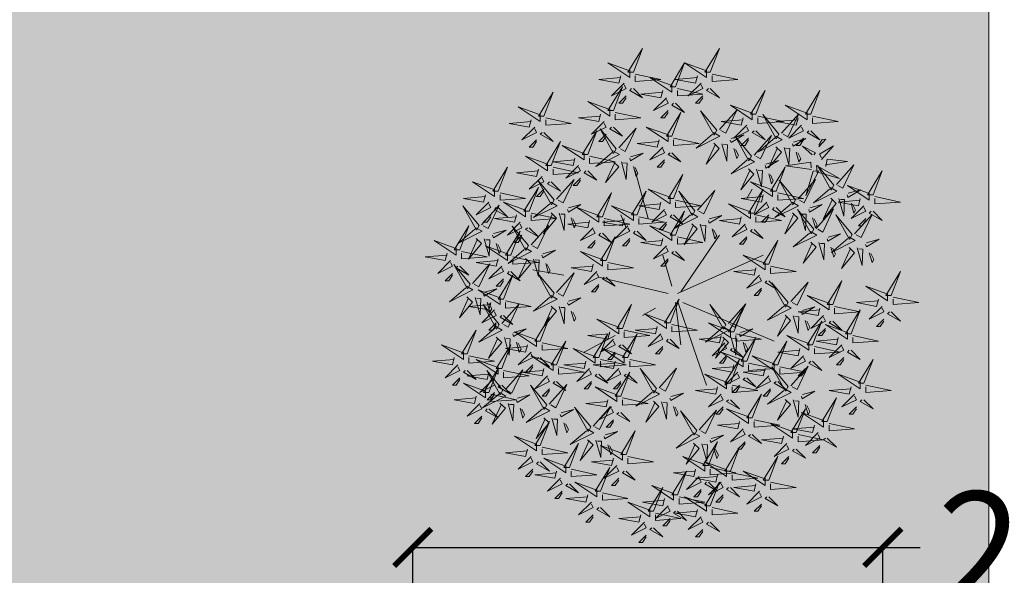
# Model space of a CAD drawing. Units: inches. Extents: x 1704 to 6393, y -157 to 1172.
# Tile 94 of 122: x 2667 to 2720, y 942 to 972. Entities that reach past the tile are written whole.
import ezdxf

# ---------------------------------------------------------------- set-up
doc = ezdxf.new("R2010")
doc.units = ezdxf.units.IN
doc.header["$MEASUREMENT"] = 0
for name, color, linetype, lineweight in [('A-ANNO-DIMS', 7, 'Continuous', 13), ('L-HRDS', 8, 'Continuous', 18), ('L-shrub', 74, 'Continuous', 18)]:
    doc.layers.add(name, color=color, linetype=linetype, lineweight=lineweight)
doc.layers.add('L-HRDS-PATT', color=9, linetype='Continuous', lineweight=13, true_color=0xc5c1ba)
doc.styles.get("Standard").update_dxf_attribs({"font": 'arial.ttf'})
doc.dimstyles.get("Standard").update_dxf_attribs({"dimtxt": 6, "dimasz": 2, "dimexe": 0.18, "dimexo": 0.0625, "dimgap": 0.09, "dimtad": 0, "dimtih": 1, "dimtoh": 1, "dimdec": 1, "dimzin": 0, "dimdsep": 46, "dimlunit": 3, "dimtxsty": 'Standard', "dimblk": 'ARCHTICK', "dimcen": 0.09, "dimadec": 0, "dimazin": 0, "dimtfac": 1, "dimtdec": 1, "dimtofl": 0, "dimtmove": 0, "dimatfit": 3, "dimfxl": 1, "dimtolj": 1, "dimtzin": 0, "dimarcsym": 0})

# ---------------------------------------------------------------- blocks, each defined once
blk = doc.blocks.new('autumn shrub')
at = {"layer": 'L-shrub'}
for p, q in [((11.5, 1.9), (51.9, 98)), ((1.9, -3.8), (-38.5, 86.5)), ((-98.1, 69.2), (-107.7, 74.9)), ((0, 0), (-59.6, 40.4)), ((71.2, 17.3), (98.1, 26.9)), ((9.6, -3.8), (71.2, 17.3)), ((11.5, -5.8), (55.8, 0)), ((-5.8, -9.6), (-38.5, -19.2)), ((1.9, -13.5), (-15.4, -86.5)), ((17.3, -26.9), (25, -40.4)), ((-77, -34.6), (-127, -48)), ((-67.3, -57.6), (-80.8, -63.4)), ((46.2, -69.2), (63.5, -101.8)), ((-17.3, -123), (-23.1, -155.6))]:
    blk.add_line(p, q, dxfattribs=at)
for points in [[(5.8, 222.9), (11.5, 249.8), (13.5, 222.9), (7.7, 222.9)], [(-100, 203.7), (-94.3, 230.6), (-92.3, 203.7), (-98.1, 203.7)], [(3.8, 221), (-21.2, 230.6), (3.8, 215.2), (3.8, 221)], [(21.2, 221), (30.8, 230.6), (23.1, 217.1), (21.2, 219)], [(98.1, 194.1), (103.9, 221), (105.8, 194.1), (100, 194.1)], [(-102, 201.8), (-127, 211.4), (-102, 196), (-102, 201.8)], [(-84.6, 201.8), (-75, 211.4), (-82.7, 197.9), (-84.6, 199.8)], [(-51.5, 195), (-55.2, 208.1), (-47.2, 194.8), (-49.8, 194)], [(1.9, 217.1), (9.6, 217.1), (-5.8, 194.1), (1.9, 215.2)], [(7.7, 207.5), (15.4, 205.6), (11.5, 184.5), (9.6, 207.5)], [(15.4, 211.4), (28.9, 197.9), (21.2, 213.3), (17.3, 211.4)], [(28.9, 213.3), (36.6, 205.6), (36.6, 209.4), (30.8, 213.3)], [(46.2, 180.6), (51.9, 207.5), (53.9, 180.6), (48.1, 180.6)], [(-103.9, 197.9), (-96.2, 197.9), (-111.6, 174.9), (-103.9, 196)], [(-60.7, 182.5), (-81.3, 200.8), (-57, 189.2), (-59.8, 184.2)], [(-41, 197.9), (-30.6, 200.8), (-33.9, 202.7), (-40.1, 199.6)], [(96.2, 192.1), (71.2, 201.8), (96.2, 186.4), (96.2, 192.1)], [(113.5, 192.1), (123.1, 201.8), (115.4, 188.3), (113.5, 190.2)], [(-103.5, 175.8), (-107.1, 188.9), (-99.2, 175.5), (-101.8, 174.8)], [(-98.1, 188.3), (-90.4, 186.4), (-94.3, 165.2), (-96.2, 188.3)], [(-90.4, 192.1), (-77, 178.7), (-84.6, 194.1), (-88.5, 192.1)], [(-77, 194.1), (-69.3, 186.4), (-69.3, 190.2), (-75, 194.1)], [(-46, 185.2), (-27.6, 190.3), (-44.8, 191.2), (-45, 186.9)], [(15.4, 161.4), (21.2, 188.3), (23.1, 161.4), (17.3, 161.4)], [(44.2, 178.7), (19.2, 188.3), (44.2, 172.9), (44.2, 178.7)], [(61.6, 178.7), (71.2, 188.3), (63.5, 174.9), (61.6, 176.8)], [(94.3, 188.3), (102, 188.3), (86.6, 165.2), (94.3, 186.4)], [(-112.7, 163.3), (-133.3, 181.5), (-108.9, 170), (-111.7, 165)], [(-93, 178.7), (-82.5, 181.6), (-85.9, 183.5), (-92, 180.4)], [(-60, 179.9), (-80.7, 162.8), (-55, 177.1), (-60, 179.9)], [(-57.6, 176.3), (-53.8, 183), (-41.3, 158.3), (-55.9, 175.4)], [(-46.4, 176.6), (-41, 182.4), (-24.4, 168.7), (-45.5, 178.3)], [(100, 178.7), (107.7, 176.8), (103.9, 155.6), (102, 178.7)], [(107.7, 182.5), (121.2, 169.1), (113.5, 184.5), (109.7, 182.5)], [(121.2, 184.5), (128.9, 176.8), (128.9, 180.6), (123.1, 184.5)], [(138.5, 155.6), (144.3, 182.5), (146.2, 155.6), (140.4, 155.6)], [(-131.5, 152.2), (-139.3, 153.6), (-137, 174.9), (-133.4, 152)], [(-125.1, 143), (-132.8, 142.5), (-119, 166.5), (-125.2, 144.9)], [(-97.9, 166), (-79.6, 171.1), (-96.8, 172), (-97, 167.7)], [(-57.3, 154.6), (-60.9, 167.7), (-53, 154.4), (-55.6, 153.7)], [(13.5, 159.5), (-11.5, 169.1), (13.5, 153.7), (13.5, 159.5)], [(30.8, 159.5), (40.4, 169.1), (32.7, 155.6), (30.8, 157.6)], [(42.3, 174.9), (50, 174.9), (34.6, 151.8), (42.3, 172.9)], [(55.8, 169.1), (69.3, 155.6), (61.6, 171), (57.7, 169.1)], [(57.7, 140.3), (63.5, 167.2), (65.4, 140.3), (59.6, 140.3)], [(69.3, 171), (77, 163.3), (77, 167.2), (71.2, 171)], [(-184.7, 138.3), (-178.9, 165.2), (-177, 138.3), (-182.8, 138.3)], [(-138.9, 147.8), (-153.3, 160.3), (-144.5, 145.5), (-140.8, 147.7)], [(-112, 160.7), (-132.6, 143.6), (-106.9, 157.8), (-112, 160.7)], [(-109.6, 157.1), (-105.8, 163.8), (-93.3, 139.1), (-107.9, 156.2)], [(-98.4, 157.4), (-92.9, 163.2), (-76.4, 149.4), (-97.4, 159.1)], [(-66.5, 142.2), (-87.1, 160.4), (-62.7, 148.9), (-65.6, 143.8)], [(-46.8, 157.5), (-36.3, 160.5), (-39.7, 162.4), (-45.9, 159.2)], [(11.5, 155.6), (19.2, 155.6), (3.8, 132.6), (11.5, 153.7)], [(48.1, 165.2), (55.8, 163.3), (51.9, 142.2), (50, 165.2)], [(136.6, 153.7), (111.6, 163.3), (136.6, 148), (136.6, 153.7)], [(153.9, 153.7), (163.5, 163.3), (155.8, 149.9), (153.9, 151.8)], [(-186.6, 136.4), (-211.6, 146), (-186.6, 130.7), (-186.6, 136.4)], [(-169.3, 136.4), (-159.7, 146), (-167.4, 132.6), (-169.3, 134.5)], [(-152.2, 144.9), (-160.4, 152.1), (-160.2, 148.2), (-154.1, 144.8)], [(-88.1, 135.4), (-91.7, 148.5), (-83.8, 135.2), (-86.4, 134.5)], [(-51.7, 144.9), (-33.4, 150), (-50.6, 150.8), (-50.8, 146.6)], [(17.3, 146), (25, 144.1), (21.2, 123), (19.2, 146)], [(25, 149.9), (38.5, 136.4), (30.8, 151.8), (26.9, 149.9)], [(55.8, 138.3), (30.8, 148), (55.8, 132.6), (55.8, 138.3)], [(38.5, 151.8), (46.2, 144.1), (46.2, 148), (40.4, 151.8)], [(73.1, 138.3), (82.7, 148), (75, 134.5), (73.1, 136.4)], [(134.7, 149.9), (142.4, 149.9), (127, 126.8), (134.7, 148)], [(148.1, 144.1), (161.6, 130.7), (153.9, 146), (150.1, 144.1)], [(150.1, 123), (155.8, 149.9), (157.8, 123), (152, 123)], [(161.6, 146), (169.3, 138.3), (169.3, 142.2), (163.5, 146)], [(-144, 137.8), (-152.9, 127.6), (-146.2, 141.5), (-144.1, 139.7)], [(-128.5, 137), (-132.4, 109.7), (-136.2, 136.4), (-130.4, 136.8)], [(-126.7, 139), (-101.1, 131.2), (-127.1, 144.8), (-126.7, 139)], [(-97.3, 122.9), (-117.9, 141.2), (-93.5, 129.6), (-96.4, 124.6)], [(-65.8, 139.5), (-86.4, 122.5), (-60.8, 136.7), (-65.8, 139.5)], [(-77.6, 138.3), (-67.1, 141.3), (-70.5, 143.1), (-76.6, 140)], [(-63.4, 136), (-59.6, 142.7), (-47.1, 117.9), (-61.7, 135)], [(-52.2, 136.3), (-46.7, 142), (-30.2, 128.3), (-51.2, 138)], [(19.7, 127.7), (16, 140.8), (24, 127.5), (21.3, 126.8)], [(30.1, 130.6), (40.6, 133.6), (37.3, 135.5), (31.1, 132.3)], [(108.2, 127.7), (104.5, 140.8), (112.5, 127.5), (109.8, 126.8)], [(118.6, 130.6), (129.1, 133.6), (125.8, 135.5), (119.6, 132.3)], [(140.4, 140.3), (148.1, 138.3), (144.3, 117.2), (142.4, 140.3)], [(-188.5, 132.6), (-180.8, 132.6), (-196.2, 109.5), (-188.5, 130.7)], [(-175.1, 126.8), (-161.6, 113.4), (-169.3, 128.7), (-173.1, 126.8)], [(-161.6, 128.7), (-153.9, 121.1), (-153.9, 124.9), (-159.7, 128.7)], [(-157.3, 118.1), (-161, 131.2), (-153, 117.9), (-155.6, 117.2)], [(-146.8, 121), (-136.4, 124), (-139.7, 125.9), (-145.9, 122.7)], [(-103.9, 101.8), (-98.1, 128.7), (-96.2, 101.8), (-102, 101.8)], [(-82.5, 125.7), (-64.2, 130.8), (-81.4, 131.6), (-81.6, 127.3)], [(10.4, 115.3), (-10.2, 133.5), (14.2, 122), (11.4, 116.9)], [(53.9, 134.5), (61.6, 134.5), (46.2, 111.4), (53.9, 132.6)], [(59.6, 124.9), (67.3, 123), (63.5, 101.8), (61.6, 124.9)], [(67.3, 128.7), (80.8, 115.3), (73.1, 130.7), (69.3, 128.7)], [(98.9, 115.3), (78.3, 133.5), (102.7, 122), (99.9, 116.9)], [(78.9, 103.8), (84.6, 130.7), (86.6, 103.8), (80.8, 103.8)], [(80.8, 130.7), (88.5, 123), (88.5, 126.8), (82.7, 130.7)], [(148.1, 121.1), (123.1, 130.7), (148.1, 115.3), (148.1, 121.1)], [(165.5, 121.1), (175.1, 130.7), (167.4, 117.2), (165.5, 119.1)], [(-166.6, 105.7), (-187.2, 123.9), (-162.8, 112.4), (-165.6, 107.3)], [(-182.8, 123), (-175.1, 121.1), (-178.9, 99.9), (-180.8, 123)], [(-151.8, 108.4), (-133.5, 113.5), (-150.6, 114.3), (-150.8, 110)], [(-96.6, 120.3), (-117.2, 103.3), (-91.5, 117.5), (-96.6, 120.3)], [(-94.2, 116.8), (-90.4, 123.5), (-77.9, 98.7), (-92.5, 115.8)], [(-83, 117.1), (-77.5, 122.8), (-61, 109.1), (-82, 118.7)], [(-26.9, 94.2), (-21.2, 121.1), (-19.2, 94.2), (-25, 94.2)], [(13.6, 109.1), (17.3, 115.8), (29.9, 91), (15.2, 108.1)], [(24.8, 109.4), (30.2, 115.1), (46.7, 101.4), (25.7, 111.1)], [(25.2, 118), (43.5, 123.1), (26.4, 123.9), (26.1, 119.7)], [(102.1, 109.1), (105.8, 115.8), (118.4, 91), (103.7, 108.1)], [(113.3, 109.4), (118.7, 115.1), (135.2, 101.4), (114.2, 111.1)], [(113.7, 118), (132, 123.1), (114.9, 123.9), (114.6, 119.7)], [(146.2, 117.2), (153.9, 117.2), (138.5, 94.2), (146.2, 115.3)], [(200.1, 94.2), (205.9, 121.1), (207.8, 94.2), (202, 94.2)], [(-184.7, 80.7), (-178.9, 107.6), (-177, 80.7), (-182.8, 80.7)], [(-163.4, 99.5), (-159.6, 106.2), (-147.1, 81.4), (-161.8, 98.5)], [(-152.2, 99.8), (-146.8, 105.5), (-130.2, 91.8), (-151.3, 101.5)], [(-105.8, 99.9), (-130.8, 109.5), (-105.8, 94.2), (-105.8, 99.9)], [(-88.5, 99.9), (-78.9, 109.5), (-86.6, 96.1), (-88.5, 98)], [(-80.8, 78.8), (-75, 105.7), (-73.1, 78.8), (-78.9, 78.8)], [(11.2, 112.6), (-9.5, 95.6), (16.2, 109.8), (11.2, 112.6)], [(77, 101.8), (51.9, 111.4), (77, 96.1), (77, 101.8)], [(99.7, 112.6), (79, 95.6), (104.7, 109.8), (99.7, 112.6)], [(94.3, 101.8), (103.9, 111.4), (96.2, 98), (94.3, 99.9)], [(134.7, 76.9), (140.4, 103.8), (142.4, 76.9), (136.6, 76.9)], [(152, 107.6), (159.7, 105.7), (155.8, 84.5), (153.9, 107.6)], [(159.7, 111.4), (173.1, 98), (165.5, 113.4), (161.6, 111.4)], [(173.1, 113.4), (180.8, 105.7), (180.8, 109.5), (175.1, 113.4)], [(-165.8, 103), (-186.5, 86), (-160.8, 100.2), (-165.8, 103)], [(-143.5, 76.8), (-164.1, 95.1), (-139.7, 83.5), (-142.5, 78.5)], [(-134.2, 89.3), (-137.9, 102.4), (-129.9, 89.1), (-132.6, 88.3)], [(-123.8, 92.2), (-113.3, 95.1), (-116.6, 97), (-122.8, 93.9)], [(-107.7, 96.1), (-100, 96.1), (-115.4, 73), (-107.7, 94.2)], [(-28.9, 92.2), (-53.9, 101.8), (-28.9, 86.5), (-28.9, 92.2)], [(-11.5, 92.2), (-1.9, 101.8), (-9.6, 88.4), (-11.5, 90.3)], [(75, 98), (82.7, 98), (67.3, 74.9), (75, 96.1)], [(75, 71.1), (80.8, 98), (82.7, 71.1), (77, 71.1)], [(88.5, 92.2), (102, 78.8), (94.3, 94.2), (90.4, 92.2)], [(102, 94.2), (109.7, 86.5), (109.7, 90.3), (103.9, 94.2)], [(198.2, 92.2), (173.1, 101.8), (198.2, 86.5), (198.2, 92.2)], [(215.5, 92.2), (225.1, 101.8), (217.4, 88.4), (215.5, 90.3)], [(-186.6, 78.8), (-211.6, 88.4), (-186.6, 73), (-186.6, 78.8)], [(-169.3, 78.8), (-159.7, 88.4), (-167.4, 74.9), (-169.3, 76.9)], [(-128.7, 79.5), (-110.4, 84.7), (-127.5, 85.5), (-127.8, 81.2)], [(-82.7, 76.9), (-107.7, 86.5), (-82.7, 71.1), (-82.7, 76.9)], [(-102, 86.5), (-94.3, 84.5), (-98.1, 63.4), (-100, 86.5)], [(-94.3, 90.3), (-80.8, 76.9), (-88.5, 92.2), (-92.3, 90.3)], [(-80.8, 92.2), (-73.1, 84.5), (-73.1, 88.4), (-78.9, 92.2)], [(-65.4, 76.9), (-55.8, 86.5), (-63.5, 73), (-65.4, 74.9)], [(-30.8, 88.4), (-23.1, 88.4), (-38.5, 65.3), (-30.8, 86.5)], [(-17.3, 82.6), (-3.8, 69.2), (-11.5, 84.5), (-15.4, 82.6)], [(-3.8, 84.5), (3.8, 76.9), (3.8, 80.7), (-1.9, 84.5)], [(44.2, 57.6), (50, 84.5), (51.9, 57.6), (46.2, 57.6)], [(80.8, 88.4), (88.5, 86.5), (84.6, 65.3), (82.7, 88.4)], [(132.7, 74.9), (107.7, 84.5), (132.7, 69.2), (132.7, 74.9)], [(150.1, 74.9), (159.7, 84.5), (152, 71.1), (150.1, 73)], [(196.2, 88.4), (203.9, 88.4), (188.5, 65.3), (196.2, 86.5)], [(209.7, 82.6), (223.2, 69.2), (215.5, 84.5), (211.6, 82.6)], [(223.2, 84.5), (230.9, 76.9), (230.9, 80.7), (225.1, 84.5)], [(-188.5, 74.9), (-180.8, 74.9), (-196.2, 51.9), (-188.5, 73)], [(-142.7, 74.2), (-163.4, 57.1), (-137.7, 71.4), (-142.7, 74.2)], [(-140.3, 70.6), (-136.6, 77.4), (-124, 52.6), (-138.7, 69.7)], [(-129.1, 71), (-123.7, 76.7), (-107.2, 63), (-128.2, 72.6)], [(-84.6, 73), (-77, 73), (-92.3, 50), (-84.6, 71.1)], [(-25, 78.8), (-17.3, 76.9), (-21.2, 55.7), (-23.1, 78.8)], [(42.8, 62.4), (39.1, 75.5), (47.1, 62.2), (44.4, 61.4)], [(73.1, 69.2), (48.1, 78.8), (73.1, 63.4), (73.1, 69.2)], [(90.4, 69.2), (100, 78.8), (92.3, 65.3), (90.4, 67.3)], [(98.1, 53.8), (103.9, 80.7), (105.8, 53.8), (100, 53.8)], [(190.5, 53.8), (196.2, 80.7), (198.2, 53.8), (192.4, 53.8)], [(202, 78.8), (209.7, 76.9), (205.9, 55.7), (203.9, 78.8)], [(-182.8, 65.3), (-175.1, 63.4), (-178.9, 42.3), (-180.8, 65.3)], [(-175.1, 69.2), (-161.6, 55.7), (-169.3, 71.1), (-173.1, 69.2)], [(-161.2, 52.8), (-164.8, 65.9), (-156.9, 52.6), (-159.5, 51.8)], [(-161.6, 71.1), (-153.9, 63.4), (-153.9, 67.3), (-159.7, 71.1)], [(-78.9, 63.4), (-71.2, 61.5), (-75, 40.4), (-77, 63.4)], [(-71.2, 67.3), (-57.7, 53.8), (-65.4, 69.2), (-69.3, 67.3)], [(-57.7, 69.2), (-50, 61.5), (-50, 65.3), (-55.8, 69.2)], [(33.5, 49.9), (12.9, 68.2), (37.3, 56.6), (34.5, 51.6)], [(42.3, 55.7), (17.3, 65.3), (42.3, 50), (42.3, 55.7)], [(53.2, 65.3), (63.7, 68.2), (60.4, 70.1), (54.2, 67)], [(59.6, 55.7), (69.3, 65.3), (61.6, 51.9), (59.6, 53.8)], [(71.2, 65.3), (78.9, 65.3), (63.5, 42.3), (71.2, 63.4)], [(130.8, 71.1), (138.5, 71.1), (123.1, 48), (130.8, 69.2)], [(144.3, 65.3), (157.8, 51.9), (150.1, 67.3), (146.2, 65.3)], [(157.8, 67.3), (165.5, 59.6), (165.5, 63.4), (159.7, 67.3)], [(-228.9, 32.7), (-223.2, 59.6), (-221.2, 32.7), (-227, 32.7)], [(-170.4, 40.3), (-191, 58.6), (-166.6, 47), (-169.5, 42)], [(-150.7, 55.7), (-140.2, 58.6), (-143.6, 60.5), (-149.7, 57.4)], [(40.4, 51.9), (48.1, 51.9), (32.7, 28.8), (40.4, 50)], [(48.3, 52.6), (66.6, 57.8), (49.5, 58.6), (49.2, 54.3)], [(96.2, 51.9), (71.2, 61.5), (96.2, 46.1), (96.2, 51.9)], [(77, 55.7), (84.6, 53.8), (80.8, 32.7), (78.9, 55.7)], [(84.6, 59.6), (98.1, 46.1), (90.4, 61.5), (86.6, 59.6)], [(98.1, 61.5), (105.8, 53.8), (105.8, 57.6), (100, 61.5)], [(113.5, 51.9), (123.1, 61.5), (115.4, 48), (113.5, 50)], [(136.6, 61.5), (144.3, 59.6), (140.4, 38.4), (138.5, 61.5)], [(188.5, 51.9), (163.5, 61.5), (188.5, 46.1), (188.5, 51.9)], [(184.7, 30.7), (190.5, 57.6), (192.4, 30.7), (186.6, 30.7)], [(205.9, 51.9), (215.5, 61.5), (207.8, 48), (205.9, 50)], [(227, 32.7), (232.8, 59.6), (234.7, 32.7), (228.9, 32.7)], [(-155.6, 43), (-137.3, 48.2), (-154.5, 49), (-154.7, 44.7)], [(-76.5, 29.7), (-80.2, 42.8), (-72.2, 29.5), (-74.8, 28.8)], [(34.3, 47.3), (13.6, 30.2), (39.3, 44.5), (34.3, 47.3)], [(36.7, 43.7), (40.4, 50.4), (53, 25.7), (38.3, 42.8)], [(46.2, 42.3), (53.9, 40.4), (50, 19.2), (48.1, 42.3)], [(47.9, 44.1), (53.3, 49.8), (69.8, 36.1), (48.8, 45.7)], [(53.9, 46.1), (67.3, 32.7), (59.6, 48), (55.8, 46.1)], [(67.3, 48), (75, 40.4), (75, 44.2), (69.3, 48)], [(94.3, 48), (102, 48), (86.6, 25), (94.3, 46.1)], [(107.7, 42.3), (121.2, 28.8), (113.5, 44.2), (109.7, 42.3)], [(121.2, 44.2), (128.9, 36.5), (128.9, 40.4), (123.1, 44.2)], [(154.3, 31.6), (150.7, 44.7), (158.6, 31.4), (156, 30.7)], [(186.6, 48), (194.3, 48), (178.9, 25), (186.6, 46.1)], [(200.1, 42.3), (213.5, 28.8), (205.9, 44.2), (202, 42.3)], [(213.5, 44.2), (221.2, 36.5), (221.2, 40.4), (215.5, 44.2)], [(-230.9, 30.7), (-255.9, 40.4), (-230.9, 25), (-230.9, 30.7)], [(-213.5, 30.7), (-203.9, 40.4), (-211.6, 26.9), (-213.5, 28.8)], [(-169.7, 37.7), (-190.3, 20.6), (-164.7, 34.9), (-169.7, 37.7)], [(-167.3, 34.1), (-163.5, 40.8), (-151, 16.1), (-165.6, 33.2)], [(-156.1, 34.4), (-150.6, 40.2), (-134.1, 26.5), (-155.1, 36.1)], [(-85.8, 17.3), (-106.4, 35.5), (-82, 24), (-84.8, 18.9)], [(-66, 32.7), (-55.6, 35.6), (-58.9, 37.5), (-65.1, 34.3)], [(100, 38.4), (107.7, 36.5), (103.9, 15.4), (102, 38.4)], [(145.1, 19.2), (124.5, 37.4), (148.9, 25.9), (146.1, 20.9)], [(182.8, 28.8), (157.8, 38.4), (182.8, 23.1), (182.8, 28.8)], [(164.8, 34.6), (175.3, 37.5), (171.9, 39.4), (165.8, 36.3)], [(192.4, 38.4), (200.1, 36.5), (196.2, 15.4), (194.3, 38.4)], [(225.1, 30.7), (200.1, 40.4), (225.1, 25), (225.1, 30.7)], [(200.1, 28.8), (209.7, 38.4), (202, 25), (200.1, 26.9)], [(242.4, 30.7), (252, 40.4), (244.3, 26.9), (242.4, 28.8)], [(-232.8, 26.9), (-225.1, 26.9), (-240.5, 3.8), (-232.8, 25)], [(-219.3, 21.1), (-205.9, 7.7), (-213.5, 23.1), (-217.4, 21.1)], [(-213.5, -3.8), (-207.8, 23.1), (-205.9, -3.8), (-211.6, -3.8)], [(-205.9, 23.1), (-198.2, 15.4), (-198.2, 19.2), (-203.9, 23.1)], [(-96.2, -5.8), (-90.4, 21.1), (-88.5, -5.8), (-94.3, -5.8)], [(-71, 20), (-52.7, 25.1), (-69.8, 26), (-70, 21.7)], [(-57.7, -3.8), (-51.9, 23.1), (-50, -3.8), (-55.8, -3.8)], [(159.9, 21.9), (178.2, 27), (161, 27.9), (160.8, 23.6)], [(180.8, 25), (188.5, 25), (173.1, 1.9), (180.8, 23.1)], [(194.3, 19.2), (207.8, 5.8), (200.1, 21.1), (196.2, 19.2)], [(207.8, 21.1), (215.5, 13.5), (215.5, 17.3), (209.7, 21.1)], [(223.2, 26.9), (230.9, 26.9), (215.5, 3.8), (223.2, 25)], [(215.5, -1.9), (221.2, 25), (223.2, -1.9), (217.4, -1.9)], [(236.6, 21.1), (250.1, 7.7), (242.4, 23.1), (238.6, 21.1)], [(250.1, 23.1), (257.8, 15.4), (257.8, 19.2), (252, 23.1)], [(-227, 17.3), (-219.3, 15.4), (-223.2, -5.8), (-225.1, 17.3)], [(-161.6, -7.7), (-155.8, 19.2), (-153.9, -7.7), (-159.7, -7.7)], [(-85, 14.6), (-105.7, -2.4), (-80, 11.8), (-85, 14.6)], [(-82.6, 11.1), (-78.8, 17.8), (-66.3, -6.9), (-81, 10.1)], [(-71.4, 11.4), (-66, 17.1), (-49.4, 3.4), (-70.5, 13.1)], [(34.6, -9.6), (40.4, 17.3), (42.3, -9.6), (36.6, -9.6)], [(145.8, 16.6), (125.2, -0.5), (150.9, 13.7), (145.8, 16.6)], [(148.2, 13), (152, 19.7), (164.5, -5), (149.9, 12.1)], [(159.4, 13.3), (164.9, 19.1), (181.4, 5.3), (160.4, 15)], [(186.6, 15.4), (194.3, 13.5), (190.5, -7.7), (188.5, 15.4)], [(228.9, 17.3), (236.6, 15.4), (232.8, -5.8), (230.9, 17.3)], [(-215.5, -5.8), (-240.5, 3.8), (-215.5, -11.5), (-215.5, -5.8)], [(-198.2, -5.8), (-188.5, 3.8), (-196.2, -9.6), (-198.2, -7.7)], [(-163.5, -9.6), (-188.5, 0), (-163.5, -15.4), (-163.5, -9.6)], [(-146.2, -9.6), (-136.6, 0), (-144.3, -13.5), (-146.2, -11.5)], [(-98.1, -7.7), (-123.1, 1.9), (-98.1, -13.5), (-98.1, -7.7)], [(-59.6, -5.8), (-84.6, 3.8), (-59.6, -11.5), (-59.6, -5.8)], [(-80.8, -7.7), (-71.2, 1.9), (-78.9, -11.5), (-80.8, -9.6)], [(-42.3, -5.8), (-32.7, 3.8), (-40.4, -9.6), (-42.3, -7.7)], [(110.1, -10.6), (106.5, 2.5), (114.4, -10.8), (111.8, -11.6)], [(213.5, -3.8), (188.5, 5.8), (213.5, -9.6), (213.5, -3.8)], [(230.9, -3.8), (240.5, 5.8), (232.8, -7.7), (230.9, -5.8)], [(232.8, -26.9), (238.6, 0), (240.5, -26.9), (234.7, -26.9)], [(-217.4, -9.6), (-209.7, -9.6), (-225.1, -32.7), (-217.4, -11.5)], [(-61.6, -9.6), (-53.9, -9.6), (-69.3, -32.7), (-61.6, -11.5)], [(32.7, -11.5), (7.7, -1.9), (32.7, -17.3), (32.7, -11.5)], [(50, -11.5), (59.6, -1.9), (51.9, -15.4), (50, -13.5)], [(100.9, -23.1), (80.3, -4.8), (104.6, -16.4), (101.8, -21.4)], [(120.6, -7.7), (131, -4.8), (127.7, -2.9), (121.5, -6)], [(211.6, -7.7), (219.3, -7.7), (203.9, -30.7), (211.6, -9.6)], [(-211.6, -19.2), (-203.9, -21.1), (-207.8, -42.3), (-209.7, -19.2)], [(-203.9, -15.4), (-190.5, -28.8), (-198.2, -13.5), (-202, -15.4)], [(-190.5, -13.5), (-182.8, -21.1), (-182.8, -17.3), (-188.5, -13.5)], [(-165.5, -13.5), (-157.8, -13.5), (-173.1, -36.5), (-165.5, -15.4)], [(-152, -19.2), (-138.5, -32.7), (-146.2, -17.3), (-150.1, -19.2)], [(-138.5, -17.3), (-130.8, -25), (-130.8, -21.1), (-136.6, -17.3)], [(-100, -11.5), (-92.3, -11.5), (-107.7, -34.6), (-100, -13.5)], [(-86.6, -17.3), (-73.1, -30.7), (-80.8, -15.4), (-84.6, -17.3)], [(-78.9, -44.2), (-73.1, -17.3), (-71.2, -44.2), (-77, -44.2)], [(-73.1, -15.4), (-65.4, -23.1), (-65.4, -19.2), (-71.2, -15.4)], [(-55.8, -19.2), (-48.1, -21.1), (-51.9, -42.3), (-53.9, -19.2)], [(-48.1, -15.4), (-34.6, -28.8), (-42.3, -13.5), (-46.2, -15.4)], [(-34.6, -13.5), (-26.9, -21.1), (-26.9, -17.3), (-32.7, -13.5)], [(30.8, -15.4), (38.5, -15.4), (23.1, -38.4), (30.8, -17.3)], [(44.2, -21.1), (57.7, -34.6), (50, -19.2), (46.2, -21.1)], [(57.7, -19.2), (65.4, -26.9), (65.4, -23.1), (59.6, -19.2)], [(115.6, -20.4), (134, -15.2), (116.8, -14.4), (116.6, -18.7)], [(230.9, -28.8), (205.9, -19.2), (230.9, -34.6), (230.9, -28.8)], [(217.4, -17.3), (225.1, -19.2), (221.2, -40.4), (219.3, -17.3)], [(225.1, -13.5), (238.6, -26.9), (230.9, -11.5), (227, -13.5)], [(238.6, -11.5), (246.3, -19.2), (246.3, -15.4), (240.5, -11.5)], [(248.2, -28.8), (257.8, -19.2), (250.1, -32.7), (248.2, -30.7)], [(-228.9, -48), (-223.2, -21.1), (-221.2, -48), (-227, -48)], [(-159.7, -23.1), (-152, -25), (-155.8, -46.1), (-157.8, -23.1)], [(-94.3, -21.1), (-86.6, -23.1), (-90.4, -44.2), (-92.3, -21.1)], [(36.6, -25), (44.2, -26.9), (40.4, -48), (38.5, -25)], [(71.2, -53.8), (77, -26.9), (78.9, -53.8), (73.1, -53.8)], [(101.6, -25.7), (80.9, -42.8), (106.6, -28.5), (101.6, -25.7)], [(104, -29.3), (107.8, -22.6), (120.3, -47.3), (105.7, -30.2)], [(115.2, -29), (120.6, -23.2), (137.2, -36.9), (116.1, -27.3)], [(173.1, -55.7), (178.9, -28.8), (180.8, -55.7), (175.1, -55.7)], [(-230.9, -50), (-255.9, -40.4), (-230.9, -55.7), (-230.9, -50)], [(-213.5, -50), (-203.9, -40.4), (-211.6, -53.8), (-213.5, -51.9)], [(-141.9, -52.9), (-145.6, -39.8), (-137.6, -53.1), (-140.3, -53.8)], [(-80.8, -46.1), (-105.8, -36.5), (-80.8, -51.9), (-80.8, -46.1)], [(-63.5, -46.1), (-53.9, -36.5), (-61.6, -50), (-63.5, -48)], [(40.4, -59.6), (46.2, -32.7), (48.1, -59.6), (42.3, -59.6)], [(111.6, -61.5), (117.4, -34.6), (119.3, -61.5), (113.5, -61.5)], [(228.9, -32.7), (236.6, -32.7), (221.2, -55.7), (228.9, -34.6)], [(242.4, -38.4), (255.9, -51.9), (248.2, -36.5), (244.3, -38.4)], [(255.9, -36.5), (263.6, -44.2), (263.6, -40.4), (257.8, -36.5)], [(-188.5, -69.2), (-182.8, -42.3), (-180.8, -69.2), (-186.6, -69.2)], [(-151.2, -65.4), (-171.8, -47.1), (-147.4, -58.7), (-150.2, -63.7)], [(-131.5, -50), (-121, -47), (-124.3, -45.2), (-130.5, -48.3)], [(-82.7, -50), (-75, -50), (-90.4, -73), (-82.7, -51.9)], [(-30.8, -76.9), (-25, -50), (-23.1, -76.9), (-28.9, -76.9)], [(69.3, -55.7), (44.2, -46.1), (69.3, -61.5), (69.3, -55.7)], [(86.6, -55.7), (96.2, -46.1), (88.5, -59.6), (86.6, -57.6)], [(171.2, -57.6), (146.2, -48), (171.2, -63.4), (171.2, -57.6)], [(188.5, -57.6), (198.2, -48), (190.5, -61.5), (188.5, -59.6)], [(234.7, -42.3), (242.4, -44.2), (238.6, -65.3), (236.6, -42.3)], [(-232.8, -53.8), (-225.1, -53.8), (-240.5, -76.9), (-232.8, -55.7)], [(-219.3, -59.6), (-205.9, -73), (-213.5, -57.6), (-217.4, -59.6)], [(-190.5, -71.1), (-215.5, -61.5), (-190.5, -76.9), (-190.5, -71.1)], [(-205.9, -57.6), (-198.2, -65.3), (-198.2, -61.5), (-203.9, -57.6)], [(-173.1, -71.1), (-163.5, -61.5), (-171.2, -74.9), (-173.1, -73)], [(-136.4, -62.6), (-118.1, -57.5), (-135.2, -56.7), (-135.5, -61)], [(-77, -80.7), (-71.2, -53.8), (-69.3, -80.7), (-75, -80.7)], [(-77, -59.6), (-69.3, -61.5), (-73.1, -82.6), (-75, -59.6)], [(-69.3, -55.7), (-55.8, -69.2), (-63.5, -53.8), (-67.3, -55.7)], [(-55.8, -53.8), (-48.1, -61.5), (-48.1, -57.6), (-53.9, -53.8)], [(38.5, -61.5), (13.5, -51.9), (38.5, -67.3), (38.5, -61.5)], [(55.8, -61.5), (65.4, -51.9), (57.7, -65.3), (55.8, -63.4)], [(67.3, -59.6), (75, -59.6), (59.6, -82.6), (67.3, -61.5)], [(71.2, -84.5), (77, -57.6), (78.9, -84.5), (73.1, -84.5)], [(109.7, -63.4), (84.6, -53.8), (109.7, -69.2), (109.7, -63.4)], [(127, -63.4), (136.6, -53.8), (128.9, -67.3), (127, -65.3)], [(169.3, -61.5), (177, -61.5), (161.6, -84.5), (169.3, -63.4)], [(211.6, -82.6), (217.4, -55.7), (219.3, -82.6), (213.5, -82.6)], [(-227, -63.4), (-219.3, -65.3), (-223.2, -86.5), (-225.1, -63.4)], [(-150.4, -68), (-171.1, -85), (-145.4, -70.8), (-150.4, -68)], [(-148, -71.5), (-144.3, -64.8), (-131.7, -89.6), (-146.4, -72.5)], [(-142.4, -96.1), (-136.6, -69.2), (-134.7, -96.1), (-140.4, -96.1)], [(-136.8, -71.2), (-131.4, -65.5), (-114.9, -79.2), (-135.9, -69.6)], [(-32.7, -78.8), (-57.7, -69.2), (-32.7, -84.5), (-32.7, -78.8)], [(-15.4, -78.8), (-5.8, -69.2), (-13.5, -82.6), (-15.4, -80.7)], [(36.6, -65.3), (44.2, -65.3), (28.9, -88.4), (36.6, -67.3)], [(50, -71.1), (63.5, -84.5), (55.8, -69.2), (51.9, -71.1)], [(63.5, -69.2), (71.2, -76.9), (71.2, -73), (65.4, -69.2)], [(73.1, -69.2), (80.8, -71.1), (77, -92.2), (75, -69.2)], [(80.8, -65.3), (94.3, -78.8), (86.6, -63.4), (82.7, -65.3)], [(94.3, -63.4), (102, -71.1), (102, -67.3), (96.2, -63.4)], [(107.7, -67.3), (115.4, -67.3), (100, -90.3), (107.7, -69.2)], [(121.2, -73), (134.7, -86.5), (127, -71.1), (123.1, -73)], [(134.7, -71.1), (142.4, -78.8), (142.4, -74.9), (136.6, -71.1)], [(150.5, -79.8), (146.9, -66.7), (154.8, -80), (152.2, -80.7)], [(161, -76.9), (171.4, -73.9), (168.1, -72.1), (161.9, -75.2)], [(175.1, -71.1), (182.8, -73), (178.9, -94.2), (177, -71.1)], [(182.8, -67.3), (196.2, -80.7), (188.5, -65.3), (184.7, -67.3)], [(196.2, -65.3), (203.9, -73), (203.9, -69.2), (198.2, -65.3)], [(-192.4, -74.9), (-184.7, -74.9), (-200.1, -98), (-192.4, -76.9)], [(-178.9, -80.7), (-165.5, -94.2), (-173.1, -78.8), (-177, -80.7)], [(-165.5, -78.8), (-157.8, -86.5), (-157.8, -82.6), (-163.5, -78.8)], [(-78.9, -82.6), (-103.9, -73), (-78.9, -88.4), (-78.9, -82.6)], [(-61.6, -82.6), (-51.9, -73), (-59.6, -86.5), (-61.6, -84.5)], [(-34.6, -82.6), (-26.9, -82.6), (-42.3, -105.7), (-34.6, -84.5)], [(42.3, -74.9), (50, -76.9), (46.2, -98), (44.2, -74.9)], [(69.3, -86.5), (44.2, -76.9), (69.3, -92.2), (69.3, -86.5)], [(86.6, -86.5), (96.2, -76.9), (88.5, -90.3), (86.6, -88.4)], [(113.5, -76.9), (121.2, -78.8), (117.4, -99.9), (115.4, -76.9)], [(141.3, -92.3), (120.7, -74), (145, -85.6), (142.2, -90.6)], [(209.7, -84.5), (184.7, -74.9), (209.7, -90.3), (209.7, -84.5)], [(227, -84.5), (236.6, -74.9), (228.9, -88.4), (227, -86.5)], [(-186.6, -84.5), (-178.9, -86.5), (-182.8, -107.6), (-184.7, -84.5)], [(-144.3, -98), (-169.3, -88.4), (-144.3, -103.8), (-144.3, -98)], [(-127, -98), (-117.4, -88.4), (-125.1, -101.8), (-127, -99.9)], [(-80.8, -86.5), (-73.1, -86.5), (-88.5, -109.5), (-80.8, -88.4)], [(-67.3, -92.2), (-53.9, -105.7), (-61.6, -90.3), (-65.4, -92.2)], [(-53.9, -90.3), (-46.2, -98), (-46.2, -94.2), (-51.9, -90.3)], [(-28.9, -92.2), (-21.2, -94.2), (-25, -115.3), (-26.9, -92.2)], [(-21.2, -88.4), (-7.7, -101.8), (-15.4, -86.5), (-19.2, -88.4)], [(-7.7, -86.5), (0, -94.2), (0, -90.3), (-5.8, -86.5)], [(67.3, -90.3), (75, -90.3), (59.6, -113.4), (67.3, -92.2)], [(144.4, -98.4), (148.2, -91.7), (160.7, -116.5), (146.1, -99.4)], [(155.6, -98.1), (161, -92.4), (177.6, -106.1), (156.5, -96.5)], [(156, -89.5), (174.4, -84.4), (157.2, -83.6), (157, -87.9)], [(186.6, -115.3), (192.4, -88.4), (194.3, -115.3), (188.5, -115.3)], [(207.8, -88.4), (215.5, -88.4), (200.1, -111.4), (207.8, -90.3)], [(221.2, -94.2), (234.7, -107.6), (227, -92.2), (223.2, -94.2)], [(234.7, -92.2), (242.4, -99.9), (242.4, -96.1), (236.6, -92.2)], [(-146.2, -101.8), (-138.5, -101.8), (-153.9, -124.9), (-146.2, -103.8)], [(-75, -96.1), (-67.3, -98), (-71.2, -119.1), (-73.1, -96.1)], [(73.1, -99.9), (80.8, -101.8), (77, -123), (75, -99.9)], [(78.9, -128.7), (84.6, -101.8), (86.6, -128.7), (80.8, -128.7)], [(80.8, -96.1), (94.3, -109.5), (86.6, -94.2), (82.7, -96.1)], [(94.3, -94.2), (102, -101.8), (102, -98), (96.2, -94.2)], [(142, -94.9), (121.3, -111.9), (147, -97.7), (142, -94.9)], [(213.5, -98), (221.2, -99.9), (217.4, -121.1), (215.5, -98)], [(-140.4, -111.4), (-132.7, -113.4), (-136.6, -134.5), (-138.5, -111.4)], [(-132.7, -107.6), (-119.3, -121.1), (-127, -105.7), (-130.8, -107.6)], [(-130.8, -134.5), (-125.1, -107.6), (-123.1, -134.5), (-128.9, -134.5)], [(-119.3, -105.7), (-111.6, -113.4), (-111.6, -109.5), (-117.4, -105.7)], [(-97.3, -130.7), (-117.9, -112.4), (-93.5, -124), (-96.4, -129)], [(-88.1, -118.2), (-91.7, -105.1), (-83.8, -118.4), (-86.4, -119.2)], [(-77.6, -115.3), (-67.1, -112.4), (-70.5, -110.5), (-76.6, -113.6)], [(0.8, -130.7), (-19.8, -112.4), (4.6, -124), (1.8, -129)], [(10.1, -118.2), (6.4, -105.1), (14.3, -118.4), (11.7, -119.2)], [(20.5, -115.3), (31, -112.4), (27.7, -110.5), (21.5, -113.6)], [(127.4, -125.9), (123.8, -112.8), (131.7, -126.1), (129.1, -126.9)], [(184.7, -117.2), (159.7, -107.6), (184.7, -123), (184.7, -117.2)], [(202, -117.2), (211.6, -107.6), (203.9, -121.1), (202, -119.1)], [(-182.8, -142.2), (-177, -115.3), (-175.1, -142.2), (-180.8, -142.2)], [(-82.5, -128), (-64.2, -122.9), (-81.4, -122), (-81.6, -126.3)], [(15.6, -128), (33.9, -122.9), (16.7, -122), (16.5, -126.3)], [(77, -130.7), (51.9, -121.1), (77, -136.4), (77, -130.7)], [(53.9, -146), (59.6, -119.1), (61.6, -146), (55.8, -146)], [(94.3, -130.7), (103.9, -121.1), (96.2, -134.5), (94.3, -132.6)], [(118.2, -138.4), (97.6, -120.1), (122, -131.7), (119.1, -136.7)], [(137.9, -123), (148.4, -120.1), (145, -118.2), (138.8, -121.3)], [(163.5, -146), (169.3, -119.1), (171.2, -146), (165.5, -146)], [(182.8, -121.1), (190.5, -121.1), (175.1, -144.1), (182.8, -123)], [(-184.7, -144.1), (-209.7, -134.5), (-184.7, -149.9), (-184.7, -144.1)], [(-167.4, -144.1), (-157.8, -134.5), (-165.5, -148), (-167.4, -146)], [(-132.7, -136.4), (-157.8, -126.8), (-132.7, -142.2), (-132.7, -136.4)], [(-96.6, -133.3), (-117.2, -150.4), (-91.5, -136.1), (-96.6, -133.3)], [(-115.4, -136.4), (-105.8, -126.8), (-113.5, -140.3), (-115.4, -138.3)], [(-94.2, -136.9), (-90.4, -130.2), (-77.9, -154.9), (-92.5, -137.8)], [(-83, -136.6), (-77.5, -130.8), (-61, -144.5), (-82, -134.9)], [(-82.7, -157.6), (-77, -130.7), (-75, -157.6), (-80.8, -157.6)], [(-40, -145.1), (-43.6, -132), (-35.7, -145.3), (-38.3, -146.1)], [(1.5, -133.3), (-19.1, -150.4), (6.6, -136.1), (1.5, -133.3)], [(3.9, -136.9), (7.7, -130.2), (20.3, -154.9), (5.6, -137.8)], [(15.2, -136.6), (20.6, -130.8), (37.1, -144.5), (16.1, -134.9)], [(75, -134.5), (82.7, -134.5), (67.3, -157.6), (75, -136.4)], [(132.9, -135.7), (151.3, -130.5), (134.1, -129.7), (133.9, -134)], [(188.5, -130.7), (196.2, -132.6), (192.4, -153.7), (190.5, -130.7)], [(196.2, -126.8), (209.7, -140.3), (202, -124.9), (198.2, -126.8)], [(209.7, -124.9), (217.4, -132.6), (217.4, -128.7), (211.6, -124.9)], [(-134.7, -140.3), (-127, -140.3), (-142.4, -163.3), (-134.7, -142.2)], [(-121.2, -146), (-107.7, -159.5), (-115.4, -144.1), (-119.3, -146)], [(-107.7, -144.1), (-100, -151.8), (-100, -148), (-105.8, -144.1)], [(-49.2, -157.6), (-69.8, -139.3), (-45.4, -150.9), (-48.3, -155.9)], [(-29.5, -142.2), (-19, -139.3), (-22.4, -137.4), (-28.5, -140.5)], [(51.9, -148), (26.9, -138.3), (51.9, -153.7), (51.9, -148)], [(69.3, -148), (78.9, -138.3), (71.2, -151.8), (69.3, -149.9)], [(80.8, -144.1), (88.5, -146), (84.6, -167.2), (82.7, -144.1)], [(88.5, -140.3), (102, -153.7), (94.3, -138.3), (90.4, -140.3)], [(118.9, -141), (98.2, -158.1), (123.9, -143.8), (118.9, -141)], [(102, -138.3), (109.7, -146), (109.7, -142.2), (103.9, -138.3)], [(121.3, -144.6), (125.1, -137.9), (137.6, -162.6), (123, -145.5)], [(132.5, -144.3), (138, -138.5), (154.5, -152.2), (133.5, -142.6)], [(161.6, -148), (136.6, -138.3), (161.6, -153.7), (161.6, -148)], [(178.9, -148), (188.5, -138.3), (180.8, -151.8), (178.9, -149.9)], [(-186.6, -148), (-178.9, -148), (-194.3, -171), (-186.6, -149.9)], [(-173.1, -153.7), (-159.7, -167.2), (-167.4, -151.8), (-171.2, -153.7)], [(-159.7, -151.8), (-152, -159.5), (-152, -155.6), (-157.8, -151.8)], [(-128.9, -149.9), (-121.2, -151.8), (-125.1, -172.9), (-127, -149.9)], [(-84.6, -159.5), (-109.7, -149.9), (-84.6, -165.2), (-84.6, -159.5)], [(-67.3, -159.5), (-57.7, -149.9), (-65.4, -163.3), (-67.3, -161.4)], [(-36.6, -176.8), (-30.8, -149.9), (-28.9, -176.8), (-34.6, -176.8)], [(-34.4, -154.9), (-16.1, -149.8), (-33.3, -148.9), (-33.5, -153.2)], [(50, -151.8), (57.7, -151.8), (42.3, -174.9), (50, -153.7)], [(159.7, -151.8), (167.4, -151.8), (152, -174.9), (159.7, -153.7)], [(-180.8, -157.6), (-173.1, -159.5), (-177, -180.6), (-178.9, -157.6)], [(-103.9, -190.2), (-98.1, -163.3), (-96.2, -190.2), (-102, -190.2)], [(-86.6, -163.3), (-78.9, -163.3), (-94.3, -186.4), (-86.6, -165.2)], [(-48.5, -160.2), (-69.1, -177.3), (-43.5, -163), (-48.5, -160.2)], [(-46.1, -163.8), (-42.3, -157.1), (-29.8, -181.8), (-44.4, -164.7)], [(-34.9, -163.5), (-29.4, -157.7), (-12.9, -171.4), (-33.9, -161.8)], [(9.6, -184.5), (15.4, -157.6), (17.3, -184.5), (11.5, -184.5)], [(42.8, -175.9), (39.1, -162.8), (47.1, -176.1), (44.4, -176.8)], [(55.8, -161.4), (63.5, -163.3), (59.6, -184.5), (57.7, -161.4)], [(63.5, -157.6), (77, -171), (69.3, -155.6), (65.4, -157.6)], [(77, -155.6), (84.6, -163.3), (84.6, -159.5), (78.9, -155.6)], [(82.7, -186.4), (88.5, -159.5), (90.4, -186.4), (84.6, -186.4)], [(112, -172), (108.4, -158.9), (116.3, -172.2), (113.7, -173)], [(122.5, -169.1), (133, -166.2), (129.6, -164.3), (123.4, -167.4)], [(165.5, -161.4), (173.1, -163.3), (169.3, -184.5), (167.4, -161.4)], [(173.1, -157.6), (186.6, -171), (178.9, -155.6), (175.1, -157.6)], [(186.6, -155.6), (194.3, -163.3), (194.3, -159.5), (188.5, -155.6)], [(-80.8, -172.9), (-73.1, -174.9), (-77, -196), (-78.9, -172.9)], [(-73.1, -169.1), (-59.6, -182.5), (-67.3, -167.2), (-71.2, -169.1)], [(-38.5, -178.7), (-63.5, -169.1), (-38.5, -184.5), (-38.5, -178.7)], [(-59.6, -167.2), (-51.9, -174.9), (-51.9, -171), (-57.7, -167.2)], [(-21.2, -178.7), (-11.5, -169.1), (-19.2, -182.5), (-21.2, -180.6)], [(33.5, -188.3), (12.9, -170.1), (37.3, -181.6), (34.5, -186.7)], [(53.2, -172.9), (63.7, -170), (60.4, -168.1), (54.2, -171.3)], [(102.8, -184.5), (82.2, -166.2), (106.6, -177.8), (103.7, -182.8)], [(107.7, -199.8), (113.5, -172.9), (115.4, -199.8), (109.7, -199.8)], [(117.5, -181.8), (135.9, -176.7), (118.7, -175.8), (118.5, -180.1)], [(-105.8, -192.1), (-130.8, -182.5), (-105.8, -197.9), (-105.8, -192.1)], [(-88.5, -192.1), (-78.9, -182.5), (-86.6, -196), (-88.5, -194.1)], [(-61.1, -197), (-64.8, -183.9), (-56.8, -197.2), (-59.5, -198)], [(-40.4, -182.5), (-32.7, -182.5), (-48.1, -205.6), (-40.4, -184.5)], [(7.7, -186.4), (-17.3, -176.8), (7.7, -192.1), (7.7, -186.4)], [(25, -186.4), (34.6, -176.8), (26.9, -190.2), (25, -188.3)], [(48.3, -185.6), (66.6, -180.5), (49.5, -179.6), (49.2, -183.9)], [(80.8, -188.3), (55.8, -178.7), (80.8, -194.1), (80.8, -188.3)], [(98.1, -188.3), (107.7, -178.7), (100, -192.1), (98.1, -190.2)], [(105.9, -190.7), (109.7, -184), (122.2, -208.7), (107.6, -191.6)], [(117.1, -190.4), (122.6, -184.6), (139.1, -198.3), (118.1, -188.7)], [(-107.7, -196), (-100, -196), (-115.4, -219), (-107.7, -197.9)], [(-70.4, -209.5), (-91, -191.2), (-66.6, -202.8), (-69.4, -207.8)], [(-50.7, -194.1), (-40.2, -191.2), (-43.5, -189.3), (-49.7, -192.4)], [(-34.6, -192.1), (-26.9, -194.1), (-30.8, -215.2), (-32.7, -192.1)], [(-26.9, -188.3), (-13.5, -201.8), (-21.2, -186.4), (-25, -188.3)], [(-13.5, -186.4), (-5.8, -194.1), (-5.8, -190.2), (-11.5, -186.4)], [(0.4, -206.6), (-3.2, -193.5), (4.7, -206.8), (2.1, -207.6)], [(5.8, -190.2), (13.5, -190.2), (-1.9, -213.3), (5.8, -192.1)], [(34.3, -191), (13.6, -208), (39.3, -193.8), (34.3, -191)], [(19.2, -196), (32.7, -209.4), (25, -194.1), (21.2, -196)], [(32.7, -194.1), (40.4, -201.8), (40.4, -197.9), (34.6, -194.1)], [(36.7, -194.5), (40.4, -187.8), (53, -212.5), (38.3, -195.5)], [(47.9, -194.2), (53.3, -188.4), (69.8, -202.2), (48.8, -192.5)], [(67.3, -222.9), (73.1, -196), (75, -222.9), (69.3, -222.9)], [(78.9, -192.1), (86.6, -192.1), (71.2, -215.2), (78.9, -194.1)], [(105.8, -201.8), (80.8, -192.1), (105.8, -207.5), (105.8, -201.8)], [(103.5, -187.1), (82.9, -204.2), (108.5, -189.9), (103.5, -187.1)], [(92.3, -197.9), (105.8, -211.4), (98.1, -196), (94.3, -197.9)], [(105.8, -196), (113.5, -203.7), (113.5, -199.8), (107.7, -196)], [(123.1, -201.8), (132.7, -192.1), (125.1, -205.6), (123.1, -203.7)], [(-102, -205.6), (-94.3, -207.5), (-98.1, -228.7), (-100, -205.6)], [(-94.3, -201.8), (-80.8, -215.2), (-88.5, -199.8), (-92.3, -201.8)], [(-80.8, -199.8), (-73.1, -207.5), (-73.1, -203.7), (-78.9, -199.8)], [(-55.6, -206.8), (-37.3, -201.6), (-54.4, -200.8), (-54.7, -205.1)], [(-42.3, -230.6), (-36.6, -203.7), (-34.6, -230.6), (-40.4, -230.6)], [(-8.8, -219.1), (-29.4, -200.8), (-5, -212.4), (-7.9, -217.4)], [(10.9, -203.7), (21.4, -200.8), (18, -198.9), (11.9, -202)], [(11.5, -199.8), (19.2, -201.8), (15.4, -222.9), (13.5, -199.8)], [(84.6, -201.8), (92.3, -203.7), (88.5, -224.8), (86.6, -201.8)], [(103.9, -205.6), (111.6, -205.6), (96.2, -228.7), (103.9, -207.5)], [(-69.6, -212.1), (-90.3, -229.2), (-64.6, -214.9), (-69.6, -212.1)], [(-67.2, -215.7), (-63.5, -208.9), (-50.9, -233.7), (-65.6, -216.6)], [(-56, -215.3), (-50.6, -209.6), (-34.1, -223.3), (-55.1, -213.7)], [(6, -216.4), (24.3, -211.2), (7.1, -210.4), (6.9, -214.7)], [(65.4, -224.8), (40.4, -215.2), (65.4, -230.6), (65.4, -224.8)], [(82.7, -224.8), (92.3, -215.2), (84.6, -228.7), (82.7, -226.7)], [(109.7, -215.2), (117.4, -217.1), (113.5, -238.3), (111.6, -215.2)], [(117.4, -211.4), (130.8, -224.8), (123.1, -209.4), (119.3, -211.4)], [(130.8, -209.4), (138.5, -217.1), (138.5, -213.3), (132.7, -209.4)], [(-44.2, -232.5), (-69.3, -222.9), (-44.2, -238.3), (-44.2, -232.5)], [(-8.1, -221.7), (-28.7, -238.8), (-3.1, -224.5), (-8.1, -221.7)], [(-26.9, -232.5), (-17.3, -222.9), (-25, -236.3), (-26.9, -234.4)], [(-5.7, -225.3), (-1.9, -218.6), (10.6, -243.3), (-4, -226.2)], [(5.5, -225), (11, -219.2), (27.5, -232.9), (6.5, -223.3)], [(-46.2, -236.3), (-38.5, -236.3), (-53.9, -259.4), (-46.2, -238.3)], [(63.5, -228.7), (71.2, -228.7), (55.8, -251.7), (63.5, -230.6)], [(77, -234.4), (90.4, -247.9), (82.7, -232.5), (78.9, -234.4)], [(90.4, -232.5), (98.1, -240.2), (98.1, -236.3), (92.3, -232.5)], [(-40.4, -245.9), (-32.7, -247.9), (-36.6, -269), (-38.5, -245.9)], [(-32.7, -242.1), (-19.2, -255.6), (-26.9, -240.2), (-30.8, -242.1)], [(-19.2, -240.2), (-11.5, -247.9), (-11.5, -244), (-17.3, -240.2)], [(69.3, -238.3), (77, -240.2), (73.1, -261.3), (71.2, -238.3)]]:
    blk.add_lwpolyline(points, dxfattribs=at)
blk = doc.blocks.new('_ArchTick')
at = {"color": 0, "linetype": 'ByBlock', "const_width": 0.15}
blk.add_lwpolyline([(-0.5, -0.5), (0.5, 0.5)], dxfattribs=at)
blk = doc.blocks.new('*D84')
at = {"layer": 'A-ANNO-DIMS', "color": 0, "lineweight": -2, "transparency": 16777216}
for p, q in [((2713.724, 939.698), (2717.812, 939.698)), ((2717.632, 939.698), (2717.632, 929.658)), ((2717.632, 913.234), (2717.632, 923.274)), ((2713.724, 913.234), (2717.812, 913.234))]:
    blk.add_line(p, q, dxfattribs=at)
at = {"layer": 'Defpoints', "color": 0, "lineweight": -3, "transparency": 16777216}
for p in [(2713.662, 939.698), (2713.662, 913.234), (2717.632, 913.234)]:
    blk.add_point(p, dxfattribs=at)
at = {"layer": 'A-ANNO-DIMS', "color": 0, "lineweight": -2, "transparency": 16777216, "xscale": 2, "yscale": 2, "zscale": 2}
for p, rotation in [((2717.632, 939.698), 90), ((2717.632, 913.234), 270)]:
    blk.add_blockref('_ArchTick', p, dxfattribs=dict(at, rotation=rotation))
at = {"layer": 'A-ANNO-DIMS', "color": 0, "transparency": 16777216, "insert": (2717.632, 926.466), "char_height": 6, "attachment_point": 5}
blk.add_mtext('\\A1;SHRUB B 26 TYP.', dxfattribs=at)
blk = doc.blocks.new('*D85')
at = {"layer": 'A-ANNO-DIMS', "color": 0, "lineweight": -2, "transparency": 16777216}
for p, q in [((2688.434, 939.761), (2688.434, 943.848)), ((2688.434, 943.668), (2713.662, 943.668)), ((2713.662, 939.761), (2713.662, 943.848)), ((2713.662, 943.668), (2715.662, 943.668))]:
    blk.add_line(p, q, dxfattribs=at)
at = {"layer": 'Defpoints', "color": 0, "lineweight": -3, "transparency": 16777216}
for p in [(2713.662, 943.668), (2688.434, 939.698), (2713.662, 939.698)]:
    blk.add_point(p, dxfattribs=at)
at = {"layer": 'A-ANNO-DIMS', "color": 0, "lineweight": -2, "transparency": 16777216, "xscale": 2, "yscale": 2, "zscale": 2, "rotation": 180}
blk.add_blockref('_ArchTick', (2688.434, 943.668), dxfattribs=at)
at = {"layer": 'A-ANNO-DIMS', "color": 0, "lineweight": -2, "transparency": 16777216, "xscale": 2, "yscale": 2, "zscale": 2}
blk.add_blockref('_ArchTick', (2713.662, 943.668), dxfattribs=at)
at = {"layer": 'A-ANNO-DIMS', "color": 0, "transparency": 16777216, "insert": (2730.406, 943.668), "char_height": 6, "attachment_point": 5}
blk.add_mtext('\\A1;25 TYP.', dxfattribs=at)
blk = doc.blocks.new('*D95')
at = {"layer": 'A-ANNO-DIMS', "color": 0, "lineweight": -2, "transparency": 16777216}
for p, q in [((2605.349, 895.275), (2605.349, 1105.287)), ((2605.349, 1105.107), (2657.907, 1105.107)), ((2723.349, 1105.107), (2670.791, 1105.107)), ((2723.349, 895.275), (2723.349, 1105.287))]:
    blk.add_line(p, q, dxfattribs=at)
at = {"layer": 'Defpoints', "color": 0, "lineweight": -3, "transparency": 16777216}
for p in [(2723.349, 1105.107), (2605.349, 895.213), (2723.349, 895.213)]:
    blk.add_point(p, dxfattribs=at)
at = {"layer": 'A-ANNO-DIMS', "color": 0, "lineweight": -2, "transparency": 16777216, "xscale": 2, "yscale": 2, "zscale": 2, "rotation": 180}
blk.add_blockref('_ArchTick', (2605.349, 1105.107), dxfattribs=at)
at = {"layer": 'A-ANNO-DIMS', "color": 0, "lineweight": -2, "transparency": 16777216, "xscale": 2, "yscale": 2, "zscale": 2}
blk.add_blockref('_ArchTick', (2723.349, 1105.107), dxfattribs=at)
at = {"layer": 'A-ANNO-DIMS', "color": 0, "transparency": 16777216, "insert": (2664.349, 1105.107), "char_height": 6, "attachment_point": 5}
blk.add_mtext('\\A1;118', dxfattribs=at)

msp = doc.modelspace()

# ---------------------------------------------------------------- hatches: boundary and pattern name
at = {"layer": 'L-HRDS-PATT', "transparency": 33554661}
h = msp.add_hatch(color=256, dxfattribs=at)
h.dxf.hatch_style = 1
h.paths.add_polyline_path([(2719.349, 1033.213), (2664.349, 1033.213), (2664.349, 895.213), (2719.349, 895.213)])
h.paths.add_polyline_path([(2719.349, 895.213), (2664.349, 895.213), (2605.349, 895.213), (2605.349, 872.213), (2719.349, 872.213)])
h.paths.add_polyline_path([(2719.349, 872.213), (2605.349, 872.213), (2605.349, 854.213), (2601.349, 854.213, -0.121066), (2618.034, 850.113), (2618.05, 850.14), (2619.349, 849.39), (2601.349, 818.213), (2605.349, 818.213), (2605.349, 794.213), (2605.349, 754.213), (2631.349, 754.213), (2631.349, 716.213), (2719.349, 716.213)])

# ---------------------------------------------------------------- linework, layer by layer
at = {"layer": 'L-HRDS'}
msp.add_line((2719.349, 5.658), (2719.349, 1033.213), dxfattribs=at)

# ---------------------------------------------------------------- block references
at = {"layer": 'L-shrub', "xscale": 0.0510581485411622, "yscale": 0.0510581485411622, "zscale": 0.0510581485411622, "rotation": 269.9999999999999}
msp.add_blockref('autumn shrub', (2702.828, 957.393), dxfattribs=at)

# ---------------------------------------------------------------- dimensions: what is measured, and where the dimension line sits
at = {"layer": 'A-ANNO-DIMS'}
dim = msp.add_linear_dim(base=(2723.349, 1105.107), p1=(2605.349, 895.213), p2=(2723.349, 895.213), dimstyle='Standard', override={"dimdec": 0, "dimlfac": 1, "dimrnd": 0, "dimzin": 0, "dimdsep": 46, "dimlunit": 2}, dxfattribs=at)
dim.commit()
dim.dimension.update_dxf_attribs({"geometry": '*D95', "text_midpoint": (2664.349, 1105.107)})
dim = msp.add_linear_dim(base=(2713.662, 943.668), p1=(2688.434, 939.698), p2=(2713.662, 939.698), text='<> TYP.', dimstyle='Standard', override={"dimdec": 0, "dimlfac": 1, "dimrnd": 0, "dimzin": 0, "dimdsep": 46, "dimlunit": 2}, dxfattribs=at)
dim.commit()
dim.dimension.update_dxf_attribs({"geometry": '*D85', "text_midpoint": (2730.406, 943.668)})
dim = msp.add_linear_dim(base=(2717.632, 913.234), p1=(2713.662, 939.698), p2=(2713.662, 913.234), angle=270, text='SHRUB B <> TYP.', dimstyle='Standard', override={"dimdec": 0, "dimlfac": 1, "dimrnd": 0, "dimzin": 0, "dimdsep": 46, "dimlunit": 2}, dxfattribs=at)
dim.commit()
dim.dimension.update_dxf_attribs({"geometry": '*D84', "text_midpoint": (2717.632, 926.466)})

doc.saveas('drawing.dxf')
